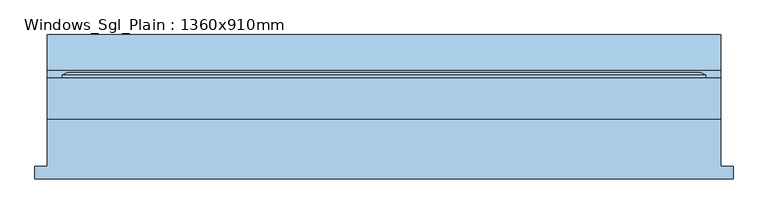
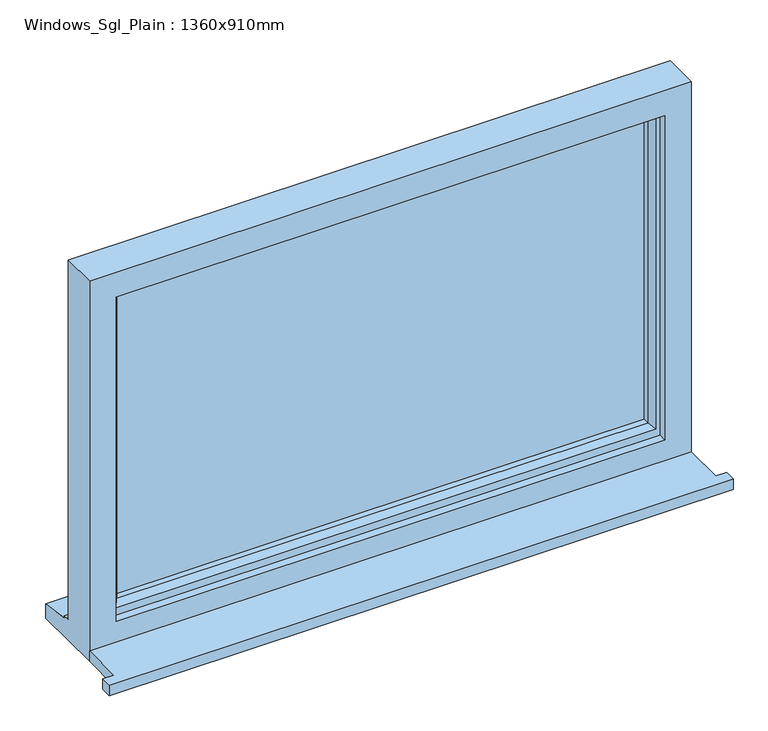
"""IFC4 building model written with IfcOpenShell, lengths in millimetres: window geometry, Windows_Sgl_Plain : 1360x910mm."""

from ifc_helpers import new_model, si_unit, frame, origin, place, context, project, spatial, polyline, outline, extrude, faceted_brep, source, transform, mapped, element, save


def windows_sgl_plain_1360x910mm_0a0c3bd6(model_context):
    return source(origin(), model_context, "Body", "SolidModel", [
        extrude(outline(polyline([(-705.0, -130.8434322), (-705.0, -105.8434322), (-680.0, -105.8434322), (-680.0, -10.2434322), (680.0, -10.2434322), (680.0, -105.8434322), (705.0, -105.8434322), (705.0, -130.8434322), (-705.0, -130.8434322)])), frame((0.0, 0.0, 1200.0), z_axis=(0.0, 0.0, 1.0), x_axis=(1.0, 0.0, 0.0)), (0.0, 0.0, 1.0), 25.0),
        faceted_brep([(-680.0, -10.2434322, 1200.0), (680.0, -10.2434322, 1200.0), (680.0, -10.2434322, 2110.0), (-680.0, -10.2434322, 2110.0), (-620.0, -10.2434322, 2050.0), (620.0, -10.2434322, 2050.0), (620.0, -10.2434322, 1275.0), (-620.0, -10.2434322, 1275.0), (-680.0, 72.7565678, 2110.0), (-680.0, 72.7565678, 1251.0), (-680.0, 87.7565678, 1249.68767), (-680.0, 87.7565678, 1244.7449676), (-680.0, 160.2565678, 1233.8088847), (-680.0, 160.2565678, 1200.0), (680.0, 72.7565678, 2110.0), (680.0, 72.7565678, 1251.0), (-640.0, 72.7565678, 2070.0), (-640.0, 72.7565678, 1263.0), (640.0, 72.7565678, 1263.0), (640.0, 72.7565678, 2070.0), (-640.0, 7.7565678, 2070.0), (-640.0, 7.7565678, 1263.0), (640.0, 7.7565678, 2070.0), (640.0, 7.7565678, 1263.0), (-620.0, 7.7565678, 2050.0), (-620.0, 7.7565678, 1275.0), (620.0, 7.7565678, 1275.0), (620.0, 7.7565678, 2050.0), (680.0, 160.2565678, 1200.0), (680.0, 160.2565678, 1233.8088847), (680.0, 87.7565678, 1244.7449676), (680.0, 87.7565678, 1249.68767)], [[[0, 1, 2, 3], [4, 5, 6, 7]], [[0, 3, 8, 9, 10, 11, 12, 13]], [[9, 8, 14, 15], [16, 17, 18, 19]], [[17, 16, 20, 21]], [[20, 22, 23, 21], [24, 25, 26, 27]], [[24, 4, 7, 25]], [[3, 2, 14, 8]], [[16, 19, 22, 20]], [[5, 4, 24, 27]], [[15, 14, 2, 1, 28, 29, 30, 31]], [[19, 18, 23, 22]], [[5, 27, 26, 6]], [[28, 1, 0, 13]], [[29, 28, 13, 12]], [[30, 29, 12, 11]], [[31, 30, 11, 10]], [[15, 31, 10, 9]], [[21, 23, 18, 17]], [[7, 6, 26, 25]]]),
        extrude(outline(polyline([(610.0, 36.7565678), (-610.0, 36.7565678), (-610.0, 60.7565678), (610.0, 60.7565678), (610.0, 36.7565678)])), frame((0.0, 0.0, 1293.0), z_axis=(0.0, 0.0, 1.0), x_axis=(1.0, 0.0, 0.0)), (0.0, 0.0, 1.0), 747.0),
        faceted_brep([(-650.0, 72.7565678, 2080.0), (-650.0, 78.5300705, 2080.0), (-650.0, 78.5300705, 1253.0), (-650.0, 72.7565678, 1253.0), (-640.0, 7.7565678, 2070.0), (-640.0, 72.7565678, 2070.0), (-640.0, 72.7565678, 1263.0), (-640.0, 7.7565678, 1263.0), (-600.0, 22.2494677, 2030.0), (-610.1480377, 7.7565678, 2040.1480377), (-610.1480377, 7.7565678, 1292.8519623), (-600.0, 22.2494677, 1303.0), (-600.0, 36.7565678, 2030.0), (-600.0, 36.7565678, 1303.0), (-610.0, 60.7565678, 2040.0), (-610.0, 36.7565678, 2040.0), (-610.0, 36.7565678, 1293.0), (-610.0, 60.7565678, 1293.0), (-600.0, 78.5300705, 2030.0), (-600.0, 60.7565678, 2030.0), (-600.0, 60.7565678, 1303.0), (-600.0, 78.5300705, 1303.0), (-617.4457548, 84.3035732, 2047.4457548), (-617.4457548, 84.3035732, 1285.5542452), (-639.2153903, 84.3035732, 2069.2153903), (-639.2153903, 84.3035732, 1263.7846097), (650.0, 78.5300705, 1253.0), (650.0, 72.7565678, 1253.0), (640.0, 72.7565678, 1263.0), (640.0, 7.7565678, 1263.0), (610.1480377, 7.7565678, 1292.8519623), (600.0, 22.2494677, 1303.0), (600.0, 36.7565678, 1303.0), (610.0, 36.7565678, 1293.0), (610.0, 60.7565678, 1293.0), (600.0, 60.7565678, 1303.0), (600.0, 78.5300705, 1303.0), (617.4457548, 84.3035732, 1285.5542452), (639.2153903, 84.3035732, 1263.7846097), (650.0, 78.5300705, 2080.0), (650.0, 72.7565678, 2080.0), (640.0, 72.7565678, 2070.0), (640.0, 7.7565678, 2070.0), (610.1480377, 7.7565678, 2040.1480377), (600.0, 22.2494677, 2030.0), (600.0, 36.7565678, 2030.0), (610.0, 36.7565678, 2040.0), (610.0, 60.7565678, 2040.0), (600.0, 60.7565678, 2030.0), (600.0, 78.5300705, 2030.0), (617.4457548, 84.3035732, 2047.4457548), (639.2153903, 84.3035732, 2069.2153903)], [[[0, 1, 2, 3]], [[4, 5, 6, 7]], [[8, 9, 10, 11]], [[12, 8, 11, 13]], [[14, 15, 16, 17]], [[18, 19, 20, 21]], [[22, 18, 21, 23]], [[1, 24, 25, 2]], [[3, 2, 26, 27]], [[7, 6, 28, 29]], [[11, 10, 30, 31]], [[13, 11, 31, 32]], [[17, 16, 33, 34]], [[21, 20, 35, 36]], [[23, 21, 36, 37]], [[2, 25, 38, 26]], [[27, 26, 39, 40]], [[29, 28, 41, 42]], [[31, 30, 43, 44]], [[32, 31, 44, 45]], [[34, 33, 46, 47]], [[36, 35, 48, 49]], [[37, 36, 49, 50]], [[26, 38, 51, 39]], [[40, 39, 1, 0]], [[3, 27, 40, 0], [5, 41, 28, 6]], [[42, 41, 5, 4]], [[7, 29, 42, 4], [9, 43, 30, 10]], [[44, 43, 9, 8]], [[45, 44, 8, 12]], [[15, 46, 33, 16], [13, 32, 45, 12]], [[47, 46, 15, 14]], [[17, 34, 47, 14], [19, 48, 35, 20]], [[49, 48, 19, 18]], [[50, 49, 18, 22]], [[24, 51, 38, 25], [23, 37, 50, 22]], [[39, 51, 24, 1]]]),
    ])


if __name__ == "__main__":
    model = new_model("IFC4")
    model_context = context("Model", 3, world=origin())
    ifc_project = project(units=[si_unit("LENGTHUNIT", "METRE", prefix="MILLI")], contexts=[model_context])
    site = spatial("IfcSite", under=ifc_project)
    building = spatial("IfcBuilding", under=site)
    placement = place(None, origin())
    windows_sgl_plain_1360x910mm_shape = windows_sgl_plain_1360x910mm_0a0c3bd6(model_context)
    element("IfcWindow", 1, ObjectType="Windows_Sgl_Plain : 1360x910mm", at=placement, inside=building, context=model_context, shape_type="MappedRepresentation", body=[
        mapped(windows_sgl_plain_1360x910mm_shape, transform((0.0, 0.0, 0.0), x_axis=(1.0, 0.0, 0.0), y_axis=(0.0, 1.0, 0.0), z_axis=(0.0, 0.0, 1.0))),
    ])
    save(model, "model.ifc")

# Revit data of these elements
# Type "Windows_Sgl_Plain : 1360x910mm"
#   Type Mark = "46"
#   Operation = "SinglePanel"
#   Construction Type Id = "SGL"
#   Manufacturer = "Revit"
#   Keynote = "L10"
#   Analytic Construction = "Large single-glazed windows"
#   Wrap Layers (Ext) from Ext = 102.5 mm
#   Wrap Layers (Int) from Ext = 177.5 mm
#   Window Board Projection = 25 mm
#   Window Board Extension = 25 mm
#   Visual Light Transmittance = 0.9
#   Solar Heat Gain Coefficient = 0.86
#   Rough Width = 1360 mm
#   Rough Height = 910 mm
#   Height = 910 mm
#   Width = 1360 mm
#   Heat Transfer Coefficient (U) = 5.5617 W/(m²·K)
#   Glazing Thickness = 24 mm
#   FrameOffset - External = 50 mm
#   Frame Depth = 65 mm
#   Default Head Height = 2110 mm
#   Cill Depth = 87.5 mm
#   Cavity Closer Width = 50 mm
#   Cavity Closer Offset from Ext = 102.5 mm
#   Cavity Closer Depth = 85 mm
#   Define Thermal Properties by = 1
#   Vis - Cavity Closers = yes
#   Define Thermal Properties by = 1
#   Material Trim = Window Frame
#   Material Glass = Glass
#   Material Frame = Window Frame
#   Wall Closure = (empty or 0)
# Element 1 (IfcWindow, "Windows_Sgl_Plain : 1360x910mm")
#   Materials on its faces: "Window Frame", "Glass"
# Materials
#   "Window Frame": colour RGB 249 249 249, transparency 0, Keynote = "L10", Cost = 0
#   "Glass": class "Glass", colour RGB 0 128 192, transparency 0.9, Description = "Soda Lime Glass", Cost = 0
